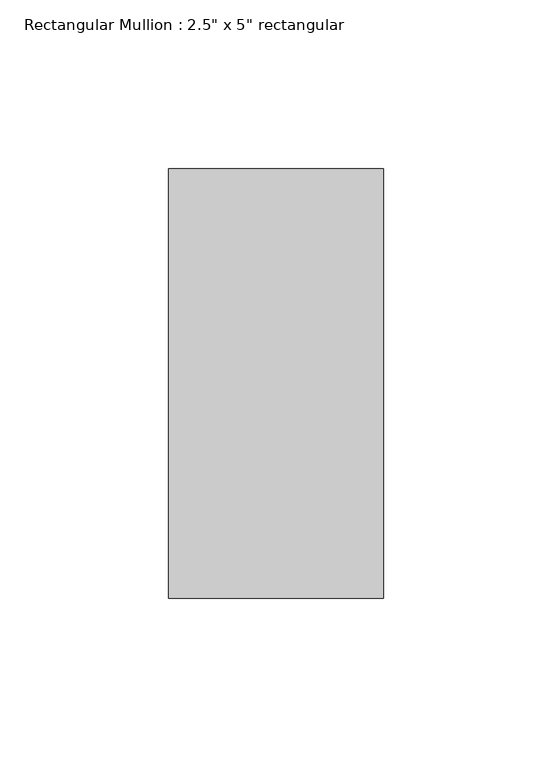
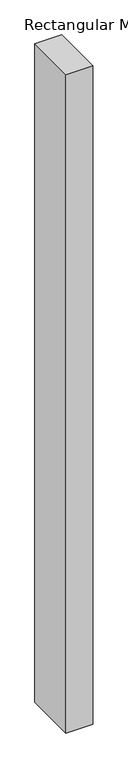
"""IFC4 building model written with IfcOpenShell, lengths in millimetres: member geometry."""

from ifc_helpers import new_model, si_unit, frame, origin, place, context, project, spatial, polyline, outline, extrude, source, transform, mapped, element, save


def member_cac0d47b(model_context):
    return source(origin(), model_context, "Body", "SweptSolid", [
        extrude(outline(polyline([(31.75, 63.5), (31.75, -63.5), (-31.75, -63.5), (-31.75, 63.5), (31.75, 63.5)])), frame((0.0, 0.0, -1649.5904225), z_axis=(0.0, 0.0, 1.0), x_axis=(1.0, 0.0, 0.0)), (0.0, 0.0, 1.0), 1649.5904225),
    ])


if __name__ == "__main__":
    model = new_model("IFC4")
    model_context = context("Model", 3, world=origin())
    ifc_project = project(units=[si_unit("LENGTHUNIT", "METRE", prefix="MILLI")], contexts=[model_context])
    site = spatial("IfcSite", under=ifc_project)
    building = spatial("IfcBuilding", under=site)
    placement = place(None, origin())
    member_shape = member_cac0d47b(model_context)
    element("IfcMember", 1, ObjectType="Rectangular Mullion : 2.5\" x 5\" rectangular", at=placement, inside=building, context=model_context, shape_type="MappedRepresentation", body=[
        mapped(member_shape, transform((0.0, 0.0, 0.0), x_axis=(1.0, 0.0, 0.0), y_axis=(0.0, 1.0, 0.0), z_axis=(0.0, 0.0, 1.0))),
    ])
    save(model, "model.ifc")

# Revit data of these elements
# Type "Rectangular Mullion : 2.5\" x 5\" rectangular"
#   built-in parameter 1007304 = 0.416667 (stored number, unit not read)
#   built-in parameter 1007301 = 0.104167 (stored number, unit not read)
#   built-in parameter 1007300 = 0.104167 (stored number, unit not read)
# Element 1 (IfcMember, "Rectangular Mullion : 2.5\" x 5\" rectangular")
#   Materials on its faces: "Aluminum"
# Materials
#   "Aluminum": class "Metal", colour RGB 247 247 247, transparency 0, Description = "Aluminum 6061", Cost = 0
